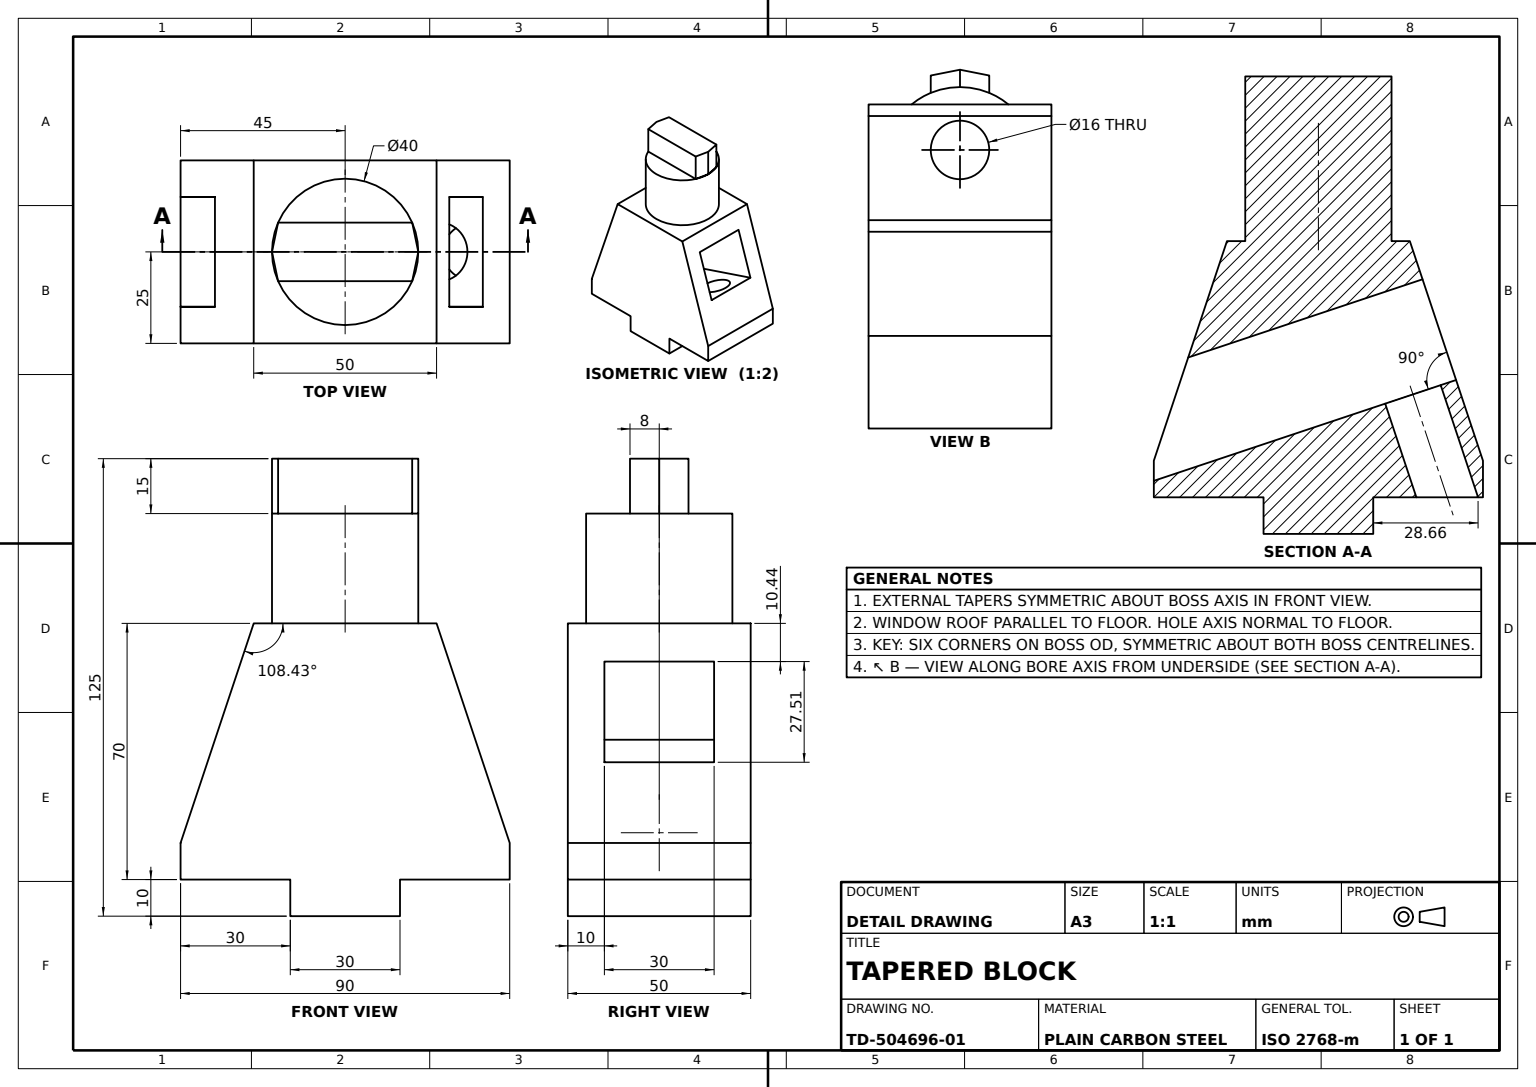
SolidWorks part; units mm, degrees
material "Plain Carbon Steel"
ref_plane "Front Plane" through (0, 0, 0) normal (0, 0, 1) x (1, 0, 0)
ref_plane "Top Plane" through (0, 0, 0) normal (0, 1, 0) x (1, 0, 0)
ref_plane "Right Plane" through (0, 0, 0) normal (1, 0, 0) x (0, 0, -1)
sketch "Base Body Profile Sketch" plane through (0, 0, 0) normal (0, 0, 1) x (1, 0, 0)
  line L0 (0, 0) -> (30, 0)
  line L1 (30, 0) -> (30, -10)
  line L2 (30, -10) -> (60, -10)
  line L3 (60, -10) -> (60, 0)
  line L4 (60, 0) -> (90, 0)
  line L5 (90, 0) -> (90, 10)
  line L6 (90, 10) -> (70, 70)
  line L7 (70, 70) -> (20, 70)
  line L8 (20, 70) -> (0, 10)
  line L9 (0, 10) -> (0, 0)
  point P3 (45, -10)
  point P12 (45, 70)
  dimension "D1" = 10
  dimension "D2" = 10
  dimension "D3" = 30
  dimension "D4" = 90
  dimension "D5" = 30
  dimension "D6" = 10
  dimension "D7" = 70
  dimension "D8" = 50
extrude "Base Body" add sketch "Base Body Profile Sketch" against normal blind 50
sketch "Side Window Sketch" plane through (84, 28, 0) normal (0.9487, 0.3162, 0) x (0, 0, -1)
  line L0 (10, 4.2719) -> (10, 33.2719)
  line L1 (10, 33.2719) -> (40, 33.2719)
  line L2 (40, 33.2719) -> (40, 4.2719)
  line L3 (40, 4.2719) -> (10, 4.2719)
  line L4 (50, 44.2719) -> (0, 44.2719) construction
  line L5 (0, -18.9737) -> (0, 44.2719) construction
  dimension "D1" = 30
  dimension "D2" = 29
  dimension "D3" = 11
  dimension "D4" = 10
extrude "Side Window Cut" cut sketch "Side Window Sketch" against normal through all
sketch "Cylindrical Boss Ø40 Sketch" plane through (0, 70, 0) normal (0, 1, 0) x (1, 0, 0)
  line L0 (20, 50) -> (20, 0) construction
  line L1 (70, 50) -> (20, 50) construction
  circle A0 centre (45, 25) radius 20
  dimension "D1" = 40
  dimension "D2" = 25
  dimension "D3" = 25
extrude "Cylindrical Boss Ø40" add sketch "Cylindrical Boss Ø40 Sketch" along normal blind 30
sketch "Top Key Sketch" plane through (0, 100, 0) normal (0, 1, 0) x (1, 0, 0)
  line L0 (25, 25) -> (65, 25) construction
  line L1 (25, 25) -> (26.6697, 33)
  line L2 (26.6697, 33) -> (63.3303, 33)
  line L3 (65, 25) -> (63.3303, 17)
  line L4 (63.3303, 17) -> (26.6697, 17)
  line L5 (26.6697, 17) -> (25, 25)
  line L6 (63.3303, 33) -> (65, 25)
  circle A0 centre (45, 25) radius 20 construction
  circle A1 centre (45, 25) radius 20 construction
  dimension "D3" = 8
  dimension "D1" = 8
  dimension "D2" = 8
extrude "Top Key" add sketch "Top Key Sketch" along normal blind 15
sketch "Hole Ø16 Sketch" plane through (-1.3509, 4.0527, 0) normal (-0.3162, 0.9487, 0) x (0.9487, 0.3162, 0)
  line L0 (88.5438, 50) -> (41.1096, 50) construction
  line L1 (41.1096, 50) -> (41.1096, 0) construction
  circle A0 centre (76.1096, 25) radius 8
  dimension "D1" = 16
  dimension "D2" = 25
  dimension "D3" = 35
extrude "Hole Ø16" cut sketch "Hole Ø16 Sketch" against normal through all
